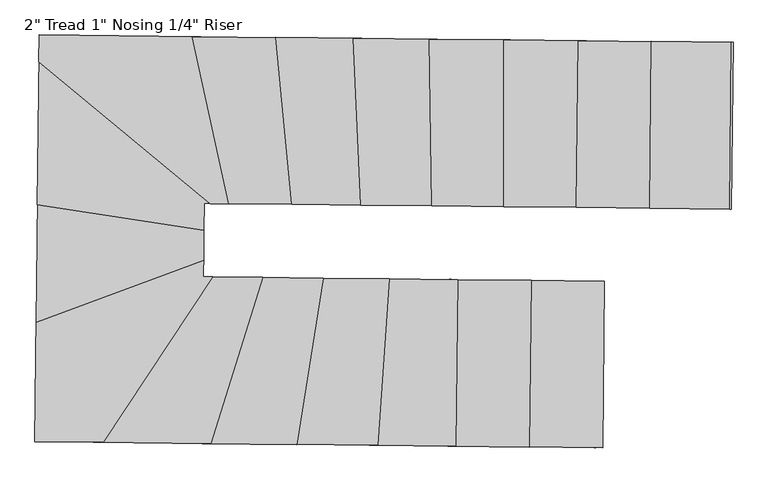
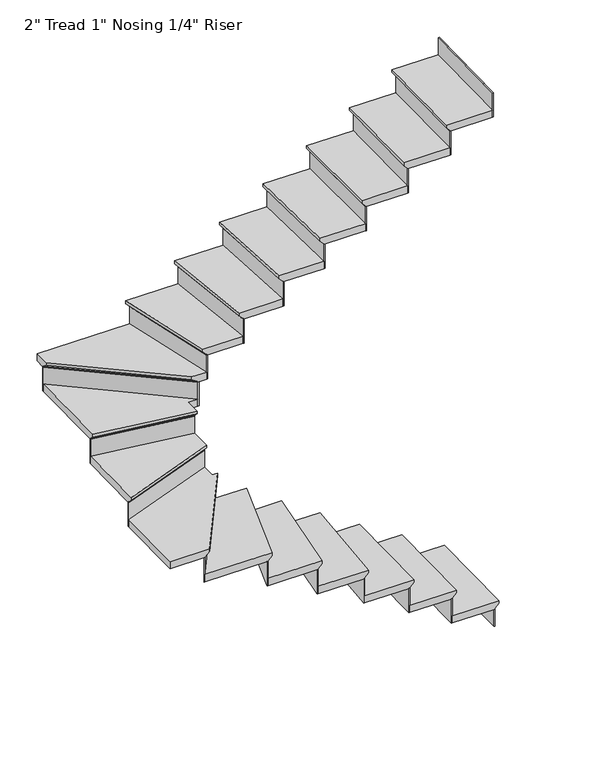
"""IFC4 building model written with IfcOpenShell, lengths in millimetres: stair flight geometry."""

from ifc_helpers import new_model, si_unit, origin, place, context, project, spatial, faceted_brep, source, transform, mapped, element, save


def stair_flight_8b4c528d(model_context):
    return source(origin(), model_context, "Body", "Brep", [
        faceted_brep([(-1961.6349602, -4965.4067295, 3350.6833333), (-1961.6349602, -4965.4067295, 3369.7333333), (-1968.4523403, -5600.3701326, 3369.7333333), (-1968.4523403, -5600.3701326, 3350.6833333), (-1987.0334963, -4965.1340343, 3325.2833333), (-1993.8508764, -5600.0974374, 3325.2833333), (-2266.4173937, -4962.134387, 3369.7333333), (-2273.2347738, -5597.0977902, 3369.7333333), (-1993.8508764, -5600.0974374, 3318.9333333), (-2273.2347738, -5597.0977902, 3318.9333333), (-2266.4173937, -4962.134387, 3318.9333333), (-1987.0334963, -4965.1340343, 3318.9333333)], [[[0, 1, 2, 3]], [[4, 0, 3, 5]], [[2, 1, 6, 7]], [[8, 9, 10, 11]], [[2, 7, 9, 8, 5, 3]], [[8, 11, 4, 5]], [[6, 1, 0, 4, 11, 10]], [[7, 6, 10, 9]]]),
        faceted_brep([(-1987.0334963, -4965.1340343, 3318.9333333), (-1987.0334963, -4965.1340343, 3200.4), (-1993.3831304, -4965.0658605, 3200.4), (-1993.3831304, -4965.0658605, 3318.9333333), (-1993.8508764, -5600.0974374, 3318.9333333), (-2000.2005104, -5600.0292636, 3318.9333333), (-2000.2005104, -5600.0292636, 3200.4), (-1993.8508764, -5600.0974374, 3200.4)], [[[0, 1, 2, 3]], [[4, 5, 6, 7]], [[1, 0, 4, 7]], [[2, 1, 7, 6]], [[3, 2, 6, 5]], [[0, 3, 5, 4]]]),
        faceted_brep([(-2266.4173937, -4962.134387, 3488.2666667), (-2266.4173937, -4962.134387, 3318.9333333), (-2272.7670277, -4962.0662132, 3318.9333333), (-2272.7670277, -4962.0662132, 3488.2666667), (-2273.2347738, -5597.0977902, 3488.2666667), (-2279.5844078, -5597.0296164, 3488.2666667), (-2279.5844078, -5597.0296164, 3318.9333333), (-2273.2347738, -5597.0977902, 3318.9333333)], [[[0, 1, 2, 3]], [[4, 5, 6, 7]], [[1, 0, 4, 7]], [[2, 1, 7, 6]], [[3, 2, 6, 5]], [[0, 3, 5, 4]]]),
        faceted_brep([(-2247.8362377, -5597.3704854, 3539.0666667), (-2241.0188576, -4962.4070822, 3539.0666667), (-2545.8012911, -4959.1347398, 3539.0666667), (-2552.6186712, -5594.0981429, 3539.0666667), (-2273.2347738, -5597.0977902, 3488.2666667), (-2552.6186712, -5594.0981429, 3488.2666667), (-2545.8012911, -4959.1347398, 3488.2666667), (-2266.4173937, -4962.134387, 3488.2666667), (-2273.2347738, -5597.0977902, 3494.6166667), (-2247.8362377, -5597.3704854, 3520.0166667), (-2266.4173937, -4962.134387, 3494.6166667), (-2241.0188576, -4962.4070822, 3520.0166667)], [[[0, 1, 2, 3]], [[4, 5, 6, 7]], [[0, 3, 5, 4, 8, 9]], [[4, 7, 10, 8]], [[2, 1, 11, 10, 7, 6]], [[3, 2, 6, 5]], [[11, 1, 0, 9]], [[10, 11, 9, 8]]]),
        faceted_brep([(-2545.8012911, -4959.1347398, 3657.6), (-2545.8012911, -4959.1347398, 3488.2666667), (-2552.1509251, -4959.066566, 3488.2666667), (-2552.1509251, -4959.066566, 3657.6), (-2552.6186712, -5594.0981429, 3657.6), (-2558.9683052, -5594.0299691, 3657.6), (-2558.9683052, -5594.0299691, 3488.2666667), (-2552.6186712, -5594.0981429, 3488.2666667)], [[[0, 1, 2, 3]], [[4, 5, 6, 7]], [[1, 0, 4, 7]], [[2, 1, 7, 6]], [[3, 2, 6, 5]], [[0, 3, 5, 4]]]),
        faceted_brep([(-2527.2201351, -5594.3708381, 3708.4), (-2520.402755, -4959.407435, 3708.4), (-2806.7760852, -4956.3327447, 3708.4), (-2850.4973934, -5590.8999232, 3708.4), (-2552.6186712, -5594.0981429, 3657.6), (-2850.4973934, -5590.8999232, 3657.6), (-2806.7760852, -4956.3327447, 3657.6), (-2545.8012911, -4959.1347398, 3657.6), (-2552.6186712, -5594.0981429, 3663.95), (-2527.2201351, -5594.3708381, 3689.35), (-2545.8012911, -4959.1347398, 3663.95), (-2520.402755, -4959.407435, 3689.35)], [[[0, 1, 2, 3]], [[4, 5, 6, 7]], [[0, 3, 5, 4, 8, 9]], [[4, 7, 10, 8]], [[2, 1, 11, 10, 7, 6]], [[3, 2, 6, 5]], [[11, 1, 0, 9]], [[10, 11, 9, 8]]]),
        faceted_brep([(-2806.7760852, -4956.3327447, 3826.9333333), (-2806.7760852, -4956.3327447, 3657.6), (-2813.1364345, -4956.2644558, 3657.6), (-2813.1364345, -4956.2644558, 3826.9333333), (-2850.4973934, -5590.8999232, 3826.9333333), (-2856.8577426, -5590.8316344, 3826.9333333), (-2856.8577426, -5590.8316344, 3657.6), (-2850.4973934, -5590.8999232, 3657.6)], [[[0, 1, 2, 3]], [[4, 5, 6, 7]], [[1, 0, 4, 7]], [[2, 1, 7, 6]], [[3, 2, 6, 5]], [[0, 3, 5, 4]]]),
        faceted_brep([(-2825.0559965, -5591.1730786, 3877.7333333), (-2781.3346883, -4956.6059001, 3877.7333333), (-3058.0757112, -4953.6346284, 3877.7333333), (-3158.4280189, -5587.5937798, 3877.7333333), (-2850.4973934, -5590.8999232, 3826.9333333), (-3158.4280189, -5587.5937798, 3826.9333333), (-3058.0757112, -4953.6346284, 3826.9333333), (-2806.7760852, -4956.3327447, 3826.9333333), (-2850.4973934, -5590.8999232, 3833.2833333), (-2825.0559965, -5591.1730786, 3858.6833333), (-2806.7760852, -4956.3327447, 3833.2833333), (-2781.3346883, -4956.6059001, 3858.6833333)], [[[0, 1, 2, 3]], [[4, 5, 6, 7]], [[0, 3, 5, 4, 8, 9]], [[4, 7, 10, 8]], [[2, 1, 11, 10, 7, 6]], [[3, 2, 6, 5]], [[11, 1, 0, 9]], [[10, 11, 9, 8]]]),
        faceted_brep([(-3058.0757112, -4953.6346284, 3996.2666667), (-3058.0757112, -4953.6346284, 3826.9333333), (-3064.4938676, -4953.5657189, 3826.9333333), (-3064.4938676, -4953.5657189, 3996.2666667), (-3158.4280189, -5587.5937798, 3996.2666667), (-3164.8461752, -5587.5248703, 3996.2666667), (-3164.8461752, -5587.5248703, 3826.9333333), (-3158.4280189, -5587.5937798, 3826.9333333)], [[[0, 1, 2, 3]], [[4, 5, 6, 7]], [[1, 0, 4, 7]], [[2, 1, 7, 6]], [[3, 2, 6, 5]], [[0, 3, 5, 4]]]),
        faceted_brep([(-3132.7553936, -5587.8694178, 4047.0666667), (-3032.4030859, -4953.9102664, 4047.0666667), (-3289.3424431, -4951.1515984, 4047.0666667), (-3487.6403792, -5584.0591417, 4047.0666667), (-3158.4280189, -5587.5937798, 3996.2666667), (-3487.6403792, -5584.0591417, 3996.2666667), (-3289.3424431, -4951.1515984, 3996.2666667), (-3058.0757112, -4953.6346284, 3996.2666667), (-3158.4280189, -5587.5937798, 4002.6166667), (-3132.7553936, -5587.8694178, 4028.0166667), (-3058.0757112, -4953.6346284, 4002.6166667), (-3032.4030859, -4953.9102664, 4028.0166667)], [[[0, 1, 2, 3]], [[4, 5, 6, 7]], [[0, 3, 5, 4, 8, 9]], [[4, 7, 10, 8]], [[2, 1, 11, 10, 7, 6]], [[3, 2, 6, 5]], [[11, 1, 0, 9]], [[10, 11, 9, 8]]]),
        faceted_brep([(-3289.3424431, -4951.1515984, 4165.6), (-3289.3424431, -4951.1515984, 3996.2666667), (-3295.9745116, -4951.0803922, 3996.2666667), (-3295.9745116, -4951.0803922, 4165.6), (-3487.6403792, -5584.0591417, 4165.6), (-3494.2724477, -5583.9879355, 4165.6), (-3494.2724477, -5583.9879355, 3996.2666667), (-3487.6403792, -5584.0591417, 3996.2666667)], [[[0, 1, 2, 3]], [[4, 5, 6, 7]], [[1, 0, 4, 7]], [[2, 1, 7, 6]], [[3, 2, 6, 5]], [[0, 3, 5, 4]]]),
        faceted_brep([(-3461.1121052, -5584.3439665, 4216.4), (-3262.8141691, -4951.4364232, 4216.4), (-3484.2219113, -4949.0592457, 4216.4), (-3900.4163626, -5579.6273103, 4216.4), (-3487.6403792, -5584.0591417, 4165.6), (-3900.4163626, -5579.6273103, 4165.6), (-3484.2219113, -4949.0592457, 4165.6), (-3289.3424431, -4951.1515984, 4165.6), (-3487.6403792, -5584.0591417, 4171.95), (-3461.1121052, -5584.3439665, 4197.35), (-3289.3424431, -4951.1515984, 4171.95), (-3262.8141691, -4951.4364232, 4197.35)], [[[0, 1, 2, 3]], [[4, 5, 6, 7]], [[0, 3, 5, 4, 8, 9]], [[4, 7, 10, 8]], [[2, 1, 11, 10, 7, 6]], [[3, 2, 6, 5]], [[11, 1, 0, 9]], [[10, 11, 9, 8]]]),
        faceted_brep([(-3484.2219113, -4949.0592457, 4334.9333333), (-3484.2219113, -4949.0592457, 4165.6), (-3491.7768309, -4948.9781311, 4165.6), (-3491.7768309, -4948.9781311, 4334.9333333), (-3900.4163626, -5579.6273103, 4334.9333333), (-3907.9712823, -5579.5461958, 4334.9333333), (-3907.9712823, -5579.5461958, 4165.6), (-3900.4163626, -5579.6273103, 4165.6)], [[[0, 1, 2, 3]], [[4, 5, 6, 7]], [[1, 0, 4, 7]], [[2, 1, 7, 6]], [[3, 2, 6, 5]], [[0, 3, 5, 4]]]),
        faceted_brep([(-4125.8898698, -5095.6676694, 4385.7333333), (-4131.0593878, -5577.1509768, 4385.7333333), (-3870.196684, -5579.9517684, 4385.7333333), (-3454.0022327, -4949.3837038, 4385.7333333), (-3489.2786045, -4949.0049537, 4385.7333333), (-3488.312708, -4859.0423992, 4385.7333333), (-4131.0593878, -5577.1509768, 4334.9333333), (-4125.8898698, -5095.6676694, 4334.9333333), (-3488.312708, -4859.0423992, 4334.9333333), (-3489.2786045, -4949.0049537, 4334.9333333), (-3484.2219113, -4949.0592457, 4334.9333333), (-3900.4163626, -5579.6273103, 4334.9333333), (-3900.4163626, -5579.6273103, 4341.2833333), (-3870.196684, -5579.9517684, 4366.6833333), (-3484.2219113, -4949.0592457, 4341.2833333), (-3454.0022327, -4949.3837038, 4366.6833333)], [[[0, 1, 2, 3, 4, 5]], [[6, 7, 8, 9, 10, 11]], [[1, 0, 7, 6]], [[2, 1, 6, 11, 12, 13]], [[11, 10, 14, 12]], [[4, 3, 15, 14, 10, 9]], [[5, 4, 9, 8]], [[0, 5, 8, 7]], [[15, 3, 2, 13]], [[14, 15, 13, 12]]]),
        faceted_brep([(-3488.312708, -4859.0423992, 4504.2666667), (-3488.312708, -4859.0423992, 4334.9333333), (-3488.2396954, -4852.2420842, 4334.9333333), (-3488.2396954, -4852.2420842, 4504.2666667), (-4125.8898698, -5095.6676694, 4504.2666667), (-4125.8168572, -5088.8673543, 4504.2666667), (-4125.8168572, -5088.8673543, 4334.9333333), (-4125.8898698, -5095.6676694, 4334.9333333)], [[[0, 1, 2, 3]], [[4, 5, 6, 7]], [[1, 0, 4, 7]], [[2, 1, 7, 6]], [[3, 2, 6, 5]], [[0, 3, 5, 4]]]),
        faceted_brep([(-4126.1819202, -5122.8689296, 4555.0666667), (-3488.6047585, -4886.2436594, 4555.0666667), (-3487.1016265, -4746.243576, 4555.0666667), (-4121.0934321, -4648.9326558, 4555.0666667), (-4125.8898698, -5095.6676694, 4504.2666667), (-4121.0934321, -4648.9326558, 4504.2666667), (-3487.1016265, -4746.243576, 4504.2666667), (-3488.312708, -4859.0423992, 4504.2666667), (-4125.8898698, -5095.6676694, 4510.6166667), (-4126.1819202, -5122.8689296, 4536.0166667), (-3488.312708, -4859.0423992, 4510.6166667), (-3488.6047585, -4886.2436594, 4536.0166667)], [[[0, 1, 2, 3]], [[4, 5, 6, 7]], [[0, 3, 5, 4, 8, 9]], [[4, 7, 10, 8]], [[3, 2, 6, 5]], [[11, 1, 0, 9]], [[10, 11, 9, 8]], [[2, 1, 11, 10, 7, 6]]]),
        faceted_brep([(-3487.1016265, -4746.243576, 4673.6), (-3487.1016265, -4746.243576, 4504.2666667), (-3487.0327638, -4739.8297815, 4504.2666667), (-3487.0327638, -4739.8297815, 4673.6), (-4121.0934321, -4648.9326558, 4673.6), (-4121.0245695, -4642.5188612, 4673.6), (-4121.0245695, -4642.5188612, 4504.2666667), (-4121.0934321, -4648.9326558, 4504.2666667)], [[[0, 1, 2, 3]], [[4, 5, 6, 7]], [[1, 0, 4, 7]], [[2, 1, 7, 6]], [[3, 2, 6, 5]], [[0, 3, 5, 4]]]),
        faceted_brep([(-4121.3688828, -4674.587834, 4724.4), (-3487.3770772, -4771.8987542, 4724.4), (-3486.2789573, -4669.6210563, 4724.4), (-3423.6180491, -4670.2938246, 4724.4), (-4115.1699262, -4097.2237198, 4724.4), (-4121.0934321, -4648.9326558, 4673.6), (-4115.1699262, -4097.2237198, 4673.6), (-3423.6180491, -4670.2938246, 4673.6), (-3486.2789573, -4669.6210563, 4673.6), (-3487.1016265, -4746.243576, 4673.6), (-4121.0934321, -4648.9326558, 4679.95), (-4121.3688828, -4674.587834, 4705.35), (-3487.1016265, -4746.243576, 4679.95), (-3487.3770772, -4771.8987542, 4705.35)], [[[0, 1, 2, 3, 4]], [[5, 6, 7, 8, 9]], [[0, 4, 6, 5, 10, 11]], [[5, 9, 12, 10]], [[2, 1, 13, 12, 9, 8]], [[4, 3, 7, 6]], [[13, 1, 0, 11]], [[12, 13, 11, 10]], [[3, 2, 8, 7]]]),
        faceted_brep([(-3423.6180491, -4670.2938246, 4842.9333333), (-3423.6180491, -4670.2938246, 4673.6), (-3413.5354356, -4670.4020781, 4673.6), (-3413.5354356, -4670.4020781, 4842.9333333), (-4115.1699262, -4097.2237198, 4842.9333333), (-4115.0821626, -4089.0495147, 4842.9333333), (-4115.0821626, -4089.0495147, 4673.6), (-4115.1699262, -4097.2237198, 4673.6)], [[[0, 1, 2, 3]], [[4, 5, 6, 7]], [[1, 0, 4, 7]], [[2, 1, 7, 6]], [[3, 2, 6, 5]], [[0, 3, 5, 4]]]),
        faceted_brep([(-3506.4342514, -4034.368057, 4893.7333333), (-4114.4249804, -4027.8402731, 4893.7333333), (-4115.5209805, -4129.9205399, 4893.7333333), (-3463.9485035, -4669.8608106, 4893.7333333), (-3365.8789969, -4670.9137486, 4893.7333333), (-4114.4249804, -4027.8402731, 4842.9333333), (-3506.4342514, -4034.368057, 4842.9333333), (-3365.8789969, -4670.9137486, 4842.9333333), (-3423.6180491, -4670.2938246, 4842.9333333), (-4115.1699262, -4097.2237198, 4842.9333333), (-3423.6180491, -4670.2938246, 4849.2833333), (-4115.1699262, -4097.2237198, 4849.2833333), (-3463.9485035, -4669.8608106, 4874.6833333), (-4115.5209805, -4129.9205399, 4874.6833333)], [[[0, 1, 2, 3, 4]], [[5, 6, 7, 8, 9]], [[1, 0, 6, 5]], [[9, 8, 10, 11]], [[4, 3, 12, 10, 8, 7]], [[0, 4, 7, 6]], [[12, 3, 2, 13]], [[10, 12, 13, 11]], [[2, 1, 5, 9, 11, 13]]]),
        faceted_brep([(-3365.8789969, -4670.9137486, 5012.2666667), (-3365.8789969, -4670.9137486, 4842.9333333), (-3359.3605829, -4670.9837346, 4842.9333333), (-3359.3605829, -4670.9837346, 5012.2666667), (-3506.4342514, -4034.368057, 5012.2666667), (-3499.9158374, -4034.438043, 5012.2666667), (-3499.9158374, -4034.438043, 4842.9333333), (-3506.4342514, -4034.368057, 4842.9333333)], [[[0, 1, 2, 3]], [[4, 5, 6, 7]], [[1, 0, 4, 7]], [[2, 1, 7, 6]], [[3, 2, 6, 5]], [[0, 3, 5, 4]]]),
        faceted_brep([(-3532.5079076, -4034.0881133, 5063.0666667), (-3391.9526531, -4670.6338049, 5063.0666667), (-3127.2086135, -4673.4762691, 5063.0666667), (-3187.4049598, -4037.793363, 5063.0666667), (-3506.4342514, -4034.368057, 5012.2666667), (-3187.4049598, -4037.793363, 5012.2666667), (-3127.2086135, -4673.4762691, 5012.2666667), (-3365.8789969, -4670.9137486, 5012.2666667), (-3506.4342514, -4034.368057, 5018.6166667), (-3532.5079076, -4034.0881133, 5044.0166667), (-3365.8789969, -4670.9137486, 5018.6166667), (-3391.9526531, -4670.6338049, 5044.0166667)], [[[0, 1, 2, 3]], [[4, 5, 6, 7]], [[0, 3, 5, 4, 8, 9]], [[4, 7, 10, 8]], [[2, 1, 11, 10, 7, 6]], [[3, 2, 6, 5]], [[11, 1, 0, 9]], [[10, 11, 9, 8]]]),
        faceted_brep([(-3127.2086135, -4673.4762691, 5181.6), (-3127.2086135, -4673.4762691, 5012.2666667), (-3120.8237144, -4673.5448215, 5012.2666667), (-3120.8237144, -4673.5448215, 5181.6), (-3187.4049598, -4037.793363, 5181.6), (-3181.0200608, -4037.8619154, 5181.6), (-3181.0200608, -4037.8619154, 5012.2666667), (-3187.4049598, -4037.793363, 5012.2666667)], [[[0, 1, 2, 3]], [[4, 5, 6, 7]], [[1, 0, 4, 7]], [[2, 1, 7, 6]], [[3, 2, 6, 5]], [[0, 3, 5, 4]]]),
        faceted_brep([(-3212.9445562, -4037.5191533, 5232.4), (-3152.7482098, -4673.2020594, 5232.4), (-2863.8799111, -4676.3035373, 5232.4), (-2892.1704009, -4040.9631932, 5232.4), (-3187.4049598, -4037.793363, 5181.6), (-2892.1704009, -4040.9631932, 5181.6), (-2863.8799111, -4676.3035373, 5181.6), (-3127.2086135, -4673.4762691, 5181.6), (-3187.4049598, -4037.793363, 5187.95), (-3212.9445562, -4037.5191533, 5213.35), (-3127.2086135, -4673.4762691, 5187.95), (-3152.7482098, -4673.2020594, 5213.35)], [[[0, 1, 2, 3]], [[4, 5, 6, 7]], [[0, 3, 5, 4, 8, 9]], [[4, 7, 10, 8]], [[2, 1, 11, 10, 7, 6]], [[3, 2, 6, 5]], [[11, 1, 0, 9]], [[10, 11, 9, 8]]]),
        faceted_brep([(-2863.8799111, -4676.3035373, 5350.9333333), (-2863.8799111, -4676.3035373, 5181.6), (-2857.5205787, -4676.3718152, 5181.6), (-2857.5205787, -4676.3718152, 5350.9333333), (-2892.1704009, -4040.9631932, 5350.9333333), (-2885.8110685, -4041.0314712, 5350.9333333), (-2885.8110685, -4041.0314712, 5181.6), (-2892.1704009, -4040.9631932, 5181.6)], [[[0, 1, 2, 3]], [[4, 5, 6, 7]], [[1, 0, 4, 7]], [[2, 1, 7, 6]], [[3, 2, 6, 5]], [[0, 3, 5, 4]]]),
        faceted_brep([(-2917.6077305, -4040.6900815, 5401.7333333), (-2889.3172407, -4676.0304256, 5401.7333333), (-2593.0867697, -4679.2109486, 5401.7333333), (-2604.2529652, -4044.0544621, 5401.7333333), (-2892.1704009, -4040.9631932, 5350.9333333), (-2604.2529652, -4044.0544621, 5350.9333333), (-2593.0867697, -4679.2109486, 5350.9333333), (-2863.8799111, -4676.3035373, 5350.9333333), (-2892.1704009, -4040.9631932, 5357.2833333), (-2917.6077305, -4040.6900815, 5382.6833333), (-2863.8799111, -4676.3035373, 5357.2833333), (-2889.3172407, -4676.0304256, 5382.6833333)], [[[0, 1, 2, 3]], [[4, 5, 6, 7]], [[0, 3, 5, 4, 8, 9]], [[4, 7, 10, 8]], [[2, 1, 11, 10, 7, 6]], [[3, 2, 6, 5]], [[11, 1, 0, 9]], [[10, 11, 9, 8]]]),
        faceted_brep([(-2593.0867697, -4679.2109486, 5520.2666667), (-2593.0867697, -4679.2109486, 5350.9333333), (-2586.7345895, -4679.2791497, 5350.9333333), (-2586.7345895, -4679.2791497, 5520.2666667), (-2604.2529652, -4044.0544621, 5520.2666667), (-2597.900785, -4044.1226632, 5520.2666667), (-2597.900785, -4044.1226632, 5350.9333333), (-2604.2529652, -4044.0544621, 5350.9333333)], [[[0, 1, 2, 3]], [[4, 5, 6, 7]], [[1, 0, 4, 7]], [[2, 1, 7, 6]], [[3, 2, 6, 5]], [[0, 3, 5, 4]]]),
        faceted_brep([(-2629.661686, -4043.7816575, 5571.0666667), (-2618.4954904, -4678.9381441, 5571.0666667), (-2319.0528449, -4682.1531551, 5571.0666667), (-2319.536107, -4047.1113675, 5571.0666667), (-2604.2529652, -4044.0544621, 5520.2666667), (-2319.536107, -4047.1113675, 5520.2666667), (-2319.0528449, -4682.1531551, 5520.2666667), (-2593.0867697, -4679.2109486, 5520.2666667), (-2604.2529652, -4044.0544621, 5526.6166667), (-2629.661686, -4043.7816575, 5552.0166667), (-2593.0867697, -4679.2109486, 5526.6166667), (-2618.4954904, -4678.9381441, 5552.0166667)], [[[0, 1, 2, 3]], [[4, 5, 6, 7]], [[0, 3, 5, 4, 8, 9]], [[4, 7, 10, 8]], [[2, 1, 11, 10, 7, 6]], [[3, 2, 6, 5]], [[11, 1, 0, 9]], [[10, 11, 9, 8]]]),
        faceted_brep([(-2319.0528449, -4682.1531551, 5689.6), (-2319.0528449, -4682.1531551, 5520.2666667), (-2312.7027912, -4682.2213334, 5520.2666667), (-2312.7027912, -4682.2213334, 5689.6), (-2319.536107, -4047.1113675, 5689.6), (-2313.1860533, -4047.1795458, 5689.6), (-2313.1860533, -4047.1795458, 5520.2666667), (-2319.536107, -4047.1113675, 5520.2666667)], [[[0, 1, 2, 3]], [[4, 5, 6, 7]], [[1, 0, 4, 7]], [[2, 1, 7, 6]], [[3, 2, 6, 5]], [[0, 3, 5, 4]]]),
        faceted_brep([(-2344.9363219, -4046.8386542, 5740.4), (-2344.4530598, -4681.8804418, 5740.4), (-2043.3209474, -4685.113592, 5740.4), (-2036.5035673, -4050.1501889, 5740.4), (-2319.536107, -4047.1113675, 5689.6), (-2036.5035673, -4050.1501889, 5689.6), (-2043.3209474, -4685.113592, 5689.6), (-2319.0528449, -4682.1531551, 5689.6), (-2319.536107, -4047.1113675, 5695.95), (-2344.9363219, -4046.8386542, 5721.35), (-2319.0528449, -4682.1531551, 5695.95), (-2344.4530598, -4681.8804418, 5721.35)], [[[0, 1, 2, 3]], [[4, 5, 6, 7]], [[0, 3, 5, 4, 8, 9]], [[4, 7, 10, 8]], [[2, 1, 11, 10, 7, 6]], [[3, 2, 6, 5]], [[11, 1, 0, 9]], [[10, 11, 9, 8]]]),
        faceted_brep([(-2043.3209474, -4685.113592, 5858.9333333), (-2043.3209474, -4685.113592, 5689.6), (-2036.9713133, -4685.1817658, 5689.6), (-2036.9713133, -4685.1817658, 5858.9333333), (-2036.5035673, -4050.1501889, 5858.9333333), (-2030.1539332, -4050.2183627, 5858.9333333), (-2030.1539332, -4050.2183627, 5689.6), (-2036.5035673, -4050.1501889, 5689.6)], [[[0, 1, 2, 3]], [[4, 5, 6, 7]], [[1, 0, 4, 7]], [[2, 1, 7, 6]], [[3, 2, 6, 5]], [[0, 3, 5, 4]]]),
        faceted_brep([(-2061.9021034, -4049.8774937, 5909.7333333), (-2068.7194835, -4684.8408968, 5909.7333333), (-1763.93705, -4688.1132393, 5909.7333333), (-1757.1196699, -4053.1498361, 5909.7333333), (-2036.5035673, -4050.1501889, 5858.9333333), (-1757.1196699, -4053.1498361, 5858.9333333), (-1763.93705, -4688.1132393, 5858.9333333), (-2043.3209474, -4685.113592, 5858.9333333), (-2036.5035673, -4050.1501889, 5865.2833333), (-2061.9021034, -4049.8774937, 5890.6833333), (-2043.3209474, -4685.113592, 5865.2833333), (-2068.7194835, -4684.8408968, 5890.6833333)], [[[0, 1, 2, 3]], [[4, 5, 6, 7]], [[0, 3, 5, 4, 8, 9]], [[4, 7, 10, 8]], [[2, 1, 11, 10, 7, 6]], [[3, 2, 6, 5]], [[11, 1, 0, 9]], [[10, 11, 9, 8]]]),
        faceted_brep([(-1763.93705, -4688.1132393, 6028.2666667), (-1763.93705, -4688.1132393, 5858.9333333), (-1757.5874159, -4688.1814131, 5858.9333333), (-1757.5874159, -4688.1814131, 6028.2666667), (-1757.1196699, -4053.1498361, 6028.2666667), (-1750.7700359, -4053.2180099, 6028.2666667), (-1750.7700359, -4053.2180099, 5858.9333333), (-1757.1196699, -4053.1498361, 5858.9333333)], [[[0, 1, 2, 3]], [[4, 5, 6, 7]], [[1, 0, 4, 7]], [[2, 1, 7, 6]], [[3, 2, 6, 5]], [[0, 3, 5, 4]]]),
        faceted_brep([(-1484.5531526, -4691.1128865, 6197.6), (-1484.5531526, -4691.1128865, 6028.2666667), (-1478.2035186, -4691.1810603, 6028.2666667), (-1478.2035186, -4691.1810603, 6197.6), (-1477.7357725, -4056.1494834, 6197.6), (-1471.3861385, -4056.2176572, 6197.6), (-1471.3861385, -4056.2176572, 6028.2666667), (-1477.7357725, -4056.1494834, 6028.2666667)], [[[0, 1, 2, 3]], [[4, 5, 6, 7]], [[1, 0, 4, 7]], [[2, 1, 7, 6]], [[3, 2, 6, 5]], [[0, 3, 5, 4]]]),
        faceted_brep([(-1782.518206, -4052.8771409, 6079.0666667), (-1789.3355861, -4687.8405441, 6079.0666667), (-1484.5531526, -4691.1128865, 6079.0666667), (-1477.7357725, -4056.1494834, 6079.0666667), (-1757.1196699, -4053.1498361, 6028.2666667), (-1477.7357725, -4056.1494834, 6028.2666667), (-1484.5531526, -4691.1128865, 6028.2666667), (-1763.93705, -4688.1132393, 6028.2666667), (-1757.1196699, -4053.1498361, 6034.6166667), (-1782.518206, -4052.8771409, 6060.0166667), (-1763.93705, -4688.1132393, 6034.6166667), (-1789.3355861, -4687.8405441, 6060.0166667)], [[[0, 1, 2, 3]], [[4, 5, 6, 7]], [[0, 3, 5, 4, 8, 9]], [[4, 7, 10, 8]], [[2, 1, 11, 10, 7, 6]], [[3, 2, 6, 5]], [[11, 1, 0, 9]], [[10, 11, 9, 8]]]),
    ])


if __name__ == "__main__":
    model = new_model("IFC4")
    model_context = context("Model", 3, world=origin())
    ifc_project = project(units=[si_unit("LENGTHUNIT", "METRE", prefix="MILLI")], contexts=[model_context])
    site = spatial("IfcSite", under=ifc_project)
    building = spatial("IfcBuilding", under=site)
    placement = place(None, origin())
    stair_flight_shape = stair_flight_8b4c528d(model_context)
    element("IfcStairFlight", 1, ObjectType="2\" Tread 1\" Nosing 1/4\" Riser", at=placement, inside=building, context=model_context, shape_type="MappedRepresentation", body=[
        mapped(stair_flight_shape, transform((0.0, 0.0, 0.0), x_axis=(1.0, 0.0, 0.0), y_axis=(0.0, 1.0, 0.0), z_axis=(0.0, 0.0, 1.0))),
    ])
    save(model, "model.ifc")
